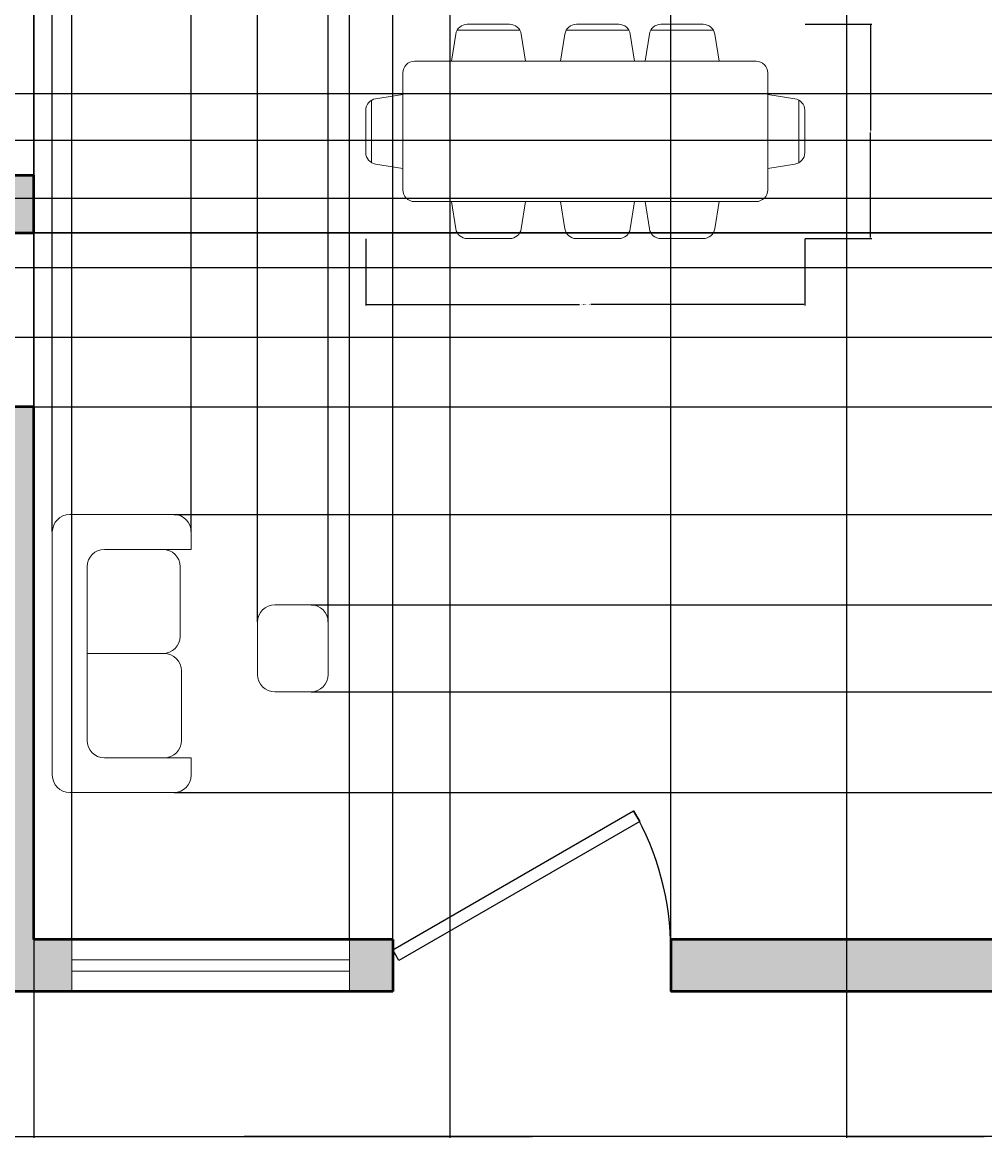
# Model space of a CAD drawing. Units: inches. Extents: x 3439 to 3988, y 1915 to 2284.
# Tile 4 of 7: x 3656 to 3822, y 1915 to 2108. Entities that reach past the tile are written whole.
import ezdxf

# ---------------------------------------------------------------- set-up
doc = ezdxf.new("R2010")
doc.units = ezdxf.units.IN
for name, color, linetype, lineweight in [('A-ANNO-DIMS', 2, 'Continuous', 18), ('A-DOOR', 3, 'Continuous', 25), ('A-FURN', 9, 'Continuous', 18), ('A-GLAZ', 4, 'Continuous', 18), ('A-WALL', 7, 'Continuous', 50)]:
    doc.layers.add(name, color=color, linetype=linetype, lineweight=lineweight)
doc.layers.add('A-WALL-PATT', color=18, linetype='Continuous', lineweight=13, true_color=0x000000)
doc.styles.get("Standard").update_dxf_attribs({"font": 'arial.ttf'})
doc.dimstyles.get("Standard").update_dxf_attribs({"dimtxt": 0.18, "dimasz": 0.18, "dimexe": 0.18, "dimexo": 0.0625, "dimgap": 0.09, "dimtad": 0, "dimtih": 1, "dimtoh": 1, "dimdec": 4, "dimzin": 0, "dimdsep": 46, "dimtxsty": 'Standard', "dimcen": 0.09, "dimadec": 0, "dimazin": 0, "dimtfac": 1, "dimtdec": 4, "dimtofl": 0, "dimtmove": 0, "dimatfit": 3, "dimfxl": 1, "dimtolj": 1, "dimtzin": 0, "dimarcsym": 0})

# ---------------------------------------------------------------- blocks, each defined once
blk = doc.blocks.new('*U4')
for p, q in [((0, 0), (0, -6)), ((40, 0), (40, -6))]:
    blk.add_line(p, q)
blk.add_lwpolyline([(0, 0), (34.64, 20), (35.52, 18.48), (0.87, -1.52)], close=True)
blk.add_arc((0, 0), 40, 0, 30)
blk = doc.blocks.new('*U5')
for p, q in [((0, 0), (0, 6)), ((40, 0), (40, 6))]:
    blk.add_line(p, q)
blk.add_lwpolyline([(0, 0), (34.64, -20), (35.52, -18.48), (0.87, 1.52)], close=True)
blk.add_arc((0, 0), 40, 330, 0)
blk = doc.blocks.new('Dining Set - 36 x 72 in.')
for p, q in [((-22.03, 26), (-5.97, 26)), ((-19.43, 27.5), (-8.57, 27.5)), ((5.97, 26), (22.03, 26)), ((8.57, 27.5), (19.43, 27.5)), ((27.65, 26), (43.71, 26)), ((30.25, 27.5), (41.11, 27.5)), ((-22.4, 24.96), (-23.48, 18)), ((-4.52, 18), (-5.6, 24.96)), ((5.6, 24.96), (4.52, 18)), ((23.48, 18), (22.4, 24.96)), ((27.29, 24.96), (26.2, 18)), ((45.17, 18), (44.08, 24.96)), ((3.02, 18), (-33, 18)), ((3.02, 18), (24.7, 18)), ((23.48, 18), (4.52, 18)), ((24.7, 18), (46.38, 18)), ((45.17, 18), (26.2, 18)), ((54.68, 18), (46.38, 18)), ((-36, 15), (-36, -15)), ((57.68, -15), (57.68, 15)), ((-42.96, 8.4), (-36, 9.48)), ((64.64, 8.4), (57.68, 9.48)), ((-44, 8.03), (-44, -8.03)), ((65.68, 8.03), (65.68, -8.03)), ((-45.5, 5.43), (-45.5, -5.43)), ((67.18, 5.43), (67.18, -5.43)), ((-36, -9.48), (-42.96, -8.4)), ((57.68, -9.48), (64.64, -8.4)), ((-33, -18), (3.02, -18)), ((-22.4, -24.96), (-23.48, -18)), ((-4.52, -18), (-5.6, -24.96)), ((3.02, -18), (24.7, -18)), ((4.52, -18), (23.48, -18)), ((5.6, -24.96), (4.52, -18)), ((23.48, -18), (22.4, -24.96)), ((24.7, -18), (46.38, -18)), ((27.29, -24.96), (26.2, -18)), ((26.2, -18), (45.17, -18)), ((45.17, -18), (44.08, -24.96)), ((46.38, -18), (54.68, -18)), ((-22.03, -26), (-5.97, -26)), ((-19.43, -27.5), (-8.57, -27.5)), ((5.97, -26), (22.03, -26)), ((8.57, -27.5), (19.43, -27.5)), ((27.65, -26), (43.71, -26)), ((30.25, -27.5), (41.11, -27.5))]:
    blk.add_line(p, q)
for centre, start, end in [((-19.43, 24.5), 90, 171.1198), ((-8.57, 24.5), 8.881, 90), ((8.57, 24.5), 90, 171.1198), ((19.43, 24.5), 8.881, 90), ((30.25, 24.5), 90, 171.1198), ((41.11, 24.5), 8.881, 90), ((-33, 15), 90, 180), ((54.68, 15), 0, 90), ((-42.5, 5.43), 98.8806, 180), ((64.18, 5.43), 0, 81.1194), ((-42.5, -5.43), 180, 261.1194), ((64.18, -5.43), 278.8806, 0), ((-33, -15), 180, 270), ((54.68, -15), 270, 0), ((-19.43, -24.5), 188.8802, 270), ((-8.57, -24.5), 270, 351.1191), ((8.57, -24.5), 188.8802, 270), ((19.43, -24.5), 270, 351.1191), ((30.25, -24.5), 188.8802, 270), ((41.11, -24.5), 270, 351.1191)]:
    blk.add_arc(centre, 3, start, end)
blk = doc.blocks.new('WINDOW-GLASS-48IN')
for p, q in [((0, 2), (48, 2)), ((0, 0), (48, 0))]:
    blk.add_line(p, q)
blk = doc.blocks.new('*D41')
at = {"layer": 'A-ANNO-DIMS', "color": 0, "lineweight": -2, "transparency": 16777216}
for p, q in [((3714.9, 2070.32), (3714.9, 2058.83)), ((3790.73, 2070.32), (3790.73, 2058.83)), ((3715.08, 2059.01), (3751.84, 2059.01)), ((3790.55, 2059.01), (3753.78, 2059.01))]:
    blk.add_line(p, q, dxfattribs=at)
at = {"layer": 'A-ANNO-DIMS', "color": 0, "transparency": 16777216}
for points in [[(3715.08, 2059.04), (3715.08, 2058.98), (3714.9, 2059.01)], [(3790.55, 2059.04), (3790.55, 2058.98), (3790.73, 2059.01)]]:
    blk.add_solid(points, dxfattribs=at)
at = {"layer": 'Defpoints', "color": 0, "transparency": 16777216}
for p in [(3714.9, 2070.38), (3790.73, 2070.38), (3790.73, 2059.01)]:
    blk.add_point(p, dxfattribs=at)
at = {"layer": 'A-ANNO-DIMS', "color": 0, "transparency": 16777216, "insert": (3752.81, 2059.01), "char_height": 0.18, "attachment_point": 5}
blk.add_mtext('\\A1;DINING SET 76', dxfattribs=at)
blk = doc.blocks.new('*D42')
at = {"layer": 'A-ANNO-DIMS', "color": 0, "lineweight": -2, "transparency": 16777216}
for p, q in [((3790.79, 2107.39), (3802.28, 2107.39)), ((3802.1, 2107.21), (3802.1, 2089.07)), ((3802.1, 2070.56), (3802.1, 2088.7)), ((3790.79, 2070.38), (3802.28, 2070.38))]:
    blk.add_line(p, q, dxfattribs=at)
at = {"layer": 'A-ANNO-DIMS', "color": 0, "transparency": 16777216}
for points in [[(3802.07, 2107.21), (3802.13, 2107.21), (3802.1, 2107.39)], [(3802.07, 2070.56), (3802.13, 2070.56), (3802.1, 2070.38)]]:
    blk.add_solid(points, dxfattribs=at)
at = {"layer": 'Defpoints', "color": 0, "transparency": 16777216}
for p in [(3790.73, 2107.39), (3802.1, 2107.39), (3790.73, 2070.38)]:
    blk.add_point(p, dxfattribs=at)
at = {"layer": 'A-ANNO-DIMS', "color": 0, "transparency": 16777216, "insert": (3802.1, 2088.89), "char_height": 0.18, "attachment_point": 5}
blk.add_mtext('\\A1;37', dxfattribs=at)
blk = doc.blocks.new('*D45')
at = {"layer": 'A-ANNO-DIMS', "color": 0, "lineweight": -2, "transparency": 16777216}
for p, q in [((3464.58, 1940.3), (3464.58, 1915.13)), ((3962.58, 1940.3), (3962.58, 1915.13)), ((3464.76, 1915.31), (3713.29, 1915.31)), ((3962.4, 1915.31), (3713.87, 1915.31))]:
    blk.add_line(p, q, dxfattribs=at)
at = {"layer": 'A-ANNO-DIMS', "color": 0, "transparency": 16777216}
for points in [[(3464.76, 1915.34), (3464.76, 1915.28), (3464.58, 1915.31)], [(3962.4, 1915.34), (3962.4, 1915.28), (3962.58, 1915.31)]]:
    blk.add_solid(points, dxfattribs=at)
at = {"layer": 'Defpoints', "color": 0, "transparency": 16777216}
for p in [(3464.58, 1940.36), (3962.58, 1940.36), (3962.58, 1915.31)]:
    blk.add_point(p, dxfattribs=at)
at = {"layer": 'A-ANNO-DIMS', "color": 0, "transparency": 16777216, "insert": (3713.58, 1915.31), "char_height": 0.18, "attachment_point": 5}
blk.add_mtext('\\A1;498', dxfattribs=at)
blk = doc.blocks.new('*D50')
at = {"layer": 'A-ANNO-DIMS', "color": 0, "lineweight": -2, "transparency": 16777216}
for p, q in [((3797.93, 2249.3), (3797.93, 1915.13)), ((3845.93, 2249.3), (3845.93, 1915.13)), ((3798.11, 1915.31), (3821.71, 1915.31)), ((3845.75, 1915.31), (3822.15, 1915.31))]:
    blk.add_line(p, q, dxfattribs=at)
at = {"layer": 'A-ANNO-DIMS', "color": 0, "transparency": 16777216}
for points in [[(3798.11, 1915.34), (3798.11, 1915.28), (3797.93, 1915.31)], [(3845.75, 1915.34), (3845.75, 1915.28), (3845.93, 1915.31)]]:
    blk.add_solid(points, dxfattribs=at)
at = {"layer": 'Defpoints', "color": 0, "transparency": 16777216}
for p in [(3797.93, 2249.36), (3845.93, 2249.36), (3845.93, 1915.31)]:
    blk.add_point(p, dxfattribs=at)
at = {"layer": 'A-ANNO-DIMS', "color": 0, "transparency": 16777216, "insert": (3821.93, 1915.31), "char_height": 0.18, "attachment_point": 5}
blk.add_mtext('\\A1;48', dxfattribs=at)
blk = doc.blocks.new('*D53')
at = {"layer": 'A-ANNO-DIMS', "color": 0, "lineweight": -2, "transparency": 16777216}
for p, q in [((3829.58, 2065.3), (3829.58, 1915.13)), ((3657.58, 2041.3), (3657.58, 1915.13)), ((3657.76, 1915.31), (3743.3, 1915.31)), ((3829.4, 1915.31), (3743.86, 1915.31))]:
    blk.add_line(p, q, dxfattribs=at)
at = {"layer": 'A-ANNO-DIMS', "color": 0, "transparency": 16777216}
for points in [[(3657.76, 1915.34), (3657.76, 1915.28), (3657.58, 1915.31)], [(3829.4, 1915.34), (3829.4, 1915.28), (3829.58, 1915.31)]]:
    blk.add_solid(points, dxfattribs=at)
at = {"layer": 'Defpoints', "color": 0, "transparency": 16777216}
for p in [(3829.58, 2065.36), (3657.58, 2041.36), (3829.58, 1915.31)]:
    blk.add_point(p, dxfattribs=at)
at = {"layer": 'A-ANNO-DIMS', "color": 0, "transparency": 16777216, "insert": (3743.58, 1915.31), "char_height": 0.18, "attachment_point": 5}
blk.add_mtext('\\A1;172', dxfattribs=at)
blk = doc.blocks.new('*D62')
at = {"layer": 'A-ANNO-DIMS', "color": 0, "lineweight": -2, "transparency": 16777216}
for p, q in [((3537.64, 2077.36), (3987.81, 2077.36)), ((3987.63, 2077.18), (3987.63, 2065.54)), ((3987.63, 2053.54), (3987.63, 2065.18)), ((3537.64, 2053.36), (3987.81, 2053.36))]:
    blk.add_line(p, q, dxfattribs=at)
at = {"layer": 'A-ANNO-DIMS', "color": 0, "transparency": 16777216}
for points in [[(3987.6, 2077.18), (3987.66, 2077.18), (3987.63, 2077.36)], [(3987.6, 2053.54), (3987.66, 2053.54), (3987.63, 2053.36)]]:
    blk.add_solid(points, dxfattribs=at)
at = {"layer": 'Defpoints', "color": 0, "transparency": 16777216}
for p in [(3537.58, 2077.36), (3987.63, 2077.36), (3537.58, 2053.36)]:
    blk.add_point(p, dxfattribs=at)
at = {"layer": 'A-ANNO-DIMS', "color": 0, "transparency": 16777216, "insert": (3987.63, 2065.36), "char_height": 0.18, "attachment_point": 5}
blk.add_mtext('\\A1;24', dxfattribs=at)
blk = doc.blocks.new('*D73')
at = {"layer": 'A-ANNO-DIMS', "color": 0, "lineweight": -2, "transparency": 16777216}
for p, q in [((3657.58, 1949.42), (3657.58, 2284)), ((3657.76, 2283.82), (3660.52, 2283.82)), ((3663.93, 2283.82), (3661.17, 2283.82)), ((3664.11, 1949.42), (3664.11, 2284))]:
    blk.add_line(p, q, dxfattribs=at)
at = {"layer": 'A-ANNO-DIMS', "color": 0, "transparency": 16777216}
for points in [[(3657.76, 2283.85), (3657.76, 2283.79), (3657.58, 2283.82)], [(3663.93, 2283.85), (3663.93, 2283.79), (3664.11, 2283.82)]]:
    blk.add_solid(points, dxfattribs=at)
at = {"layer": 'Defpoints', "color": 0, "transparency": 16777216}
for p in [(3664.11, 2283.82), (3657.58, 1949.36), (3664.11, 1949.36)]:
    blk.add_point(p, dxfattribs=at)
at = {"layer": 'A-ANNO-DIMS', "color": 0, "transparency": 16777216, "insert": (3660.85, 2283.82), "char_height": 0.18, "attachment_point": 5}
blk.add_mtext('\\A1;6.53', dxfattribs=at)
blk = doc.blocks.new('*D74')
at = {"layer": 'A-ANNO-DIMS', "color": 0, "lineweight": -2, "transparency": 16777216}
for p, q in [((3712.11, 1949.42), (3712.11, 2284)), ((3712.29, 2283.82), (3715.52, 2283.82)), ((3719.4, 2283.82), (3716.17, 2283.82)), ((3719.58, 1949.42), (3719.58, 2284))]:
    blk.add_line(p, q, dxfattribs=at)
at = {"layer": 'A-ANNO-DIMS', "color": 0, "transparency": 16777216}
for points in [[(3712.29, 2283.85), (3712.29, 2283.79), (3712.11, 2283.82)], [(3719.4, 2283.85), (3719.4, 2283.79), (3719.58, 2283.82)]]:
    blk.add_solid(points, dxfattribs=at)
at = {"layer": 'Defpoints', "color": 0, "transparency": 16777216}
for p in [(3719.58, 2283.82), (3712.11, 1949.36), (3719.58, 1949.36)]:
    blk.add_point(p, dxfattribs=at)
at = {"layer": 'A-ANNO-DIMS', "color": 0, "transparency": 16777216, "insert": (3715.85, 2283.82), "char_height": 0.18, "attachment_point": 5}
blk.add_mtext('\\A1;7.47', dxfattribs=at)
blk = doc.blocks.new('*D75')
at = {"layer": 'A-ANNO-DIMS', "color": 0, "lineweight": -2, "transparency": 16777216}
for p, q in [((3719.58, 1949.42), (3719.58, 2284)), ((3719.76, 2283.82), (3743.36, 2283.82)), ((3767.4, 2283.82), (3743.8, 2283.82)), ((3767.58, 1949.42), (3767.58, 2284))]:
    blk.add_line(p, q, dxfattribs=at)
at = {"layer": 'A-ANNO-DIMS', "color": 0, "transparency": 16777216}
for points in [[(3719.76, 2283.85), (3719.76, 2283.79), (3719.58, 2283.82)], [(3767.4, 2283.85), (3767.4, 2283.79), (3767.58, 2283.82)]]:
    blk.add_solid(points, dxfattribs=at)
at = {"layer": 'Defpoints', "color": 0, "transparency": 16777216}
for p in [(3767.58, 2283.82), (3719.58, 1949.36), (3767.58, 1949.36)]:
    blk.add_point(p, dxfattribs=at)
at = {"layer": 'A-ANNO-DIMS', "color": 0, "transparency": 16777216, "insert": (3743.58, 2283.82), "char_height": 0.18, "attachment_point": 5}
blk.add_mtext('\\A1;48', dxfattribs=at)
blk = doc.blocks.new('*D83')
at = {"layer": 'A-ANNO-DIMS', "color": 0, "lineweight": -2, "transparency": 16777216}
for p, q in [((3537.64, 2111.36), (3987.81, 2111.36)), ((3987.63, 2111.18), (3987.63, 2099.54)), ((3987.63, 2087.54), (3987.63, 2099.18)), ((3537.64, 2087.36), (3987.81, 2087.36))]:
    blk.add_line(p, q, dxfattribs=at)
at = {"layer": 'A-ANNO-DIMS', "color": 0, "transparency": 16777216}
for points in [[(3987.6, 2111.18), (3987.66, 2111.18), (3987.63, 2111.36)], [(3987.6, 2087.54), (3987.66, 2087.54), (3987.63, 2087.36)]]:
    blk.add_solid(points, dxfattribs=at)
at = {"layer": 'Defpoints', "color": 0, "transparency": 16777216}
for p in [(3537.58, 2111.36), (3987.63, 2111.36), (3537.58, 2087.36)]:
    blk.add_point(p, dxfattribs=at)
at = {"layer": 'A-ANNO-DIMS', "color": 0, "transparency": 16777216, "insert": (3987.63, 2099.36), "char_height": 0.18, "attachment_point": 5}
blk.add_mtext('\\A1;24', dxfattribs=at)
blk = doc.blocks.new('*D88')
at = {"layer": 'A-ANNO-DIMS', "color": 0, "lineweight": -2, "transparency": 16777216}
for p, q in [((3653.64, 2077.36), (3987.81, 2077.36)), ((3987.63, 2077.18), (3987.63, 2074.54)), ((3987.63, 2071.54), (3987.63, 2074.18)), ((3653.64, 2071.36), (3987.81, 2071.36))]:
    blk.add_line(p, q, dxfattribs=at)
at = {"layer": 'A-ANNO-DIMS', "color": 0, "transparency": 16777216}
for points in [[(3987.6, 2077.18), (3987.66, 2077.18), (3987.63, 2077.36)], [(3987.6, 2071.54), (3987.66, 2071.54), (3987.63, 2071.36)]]:
    blk.add_solid(points, dxfattribs=at)
at = {"layer": 'Defpoints', "color": 0, "transparency": 16777216}
for p in [(3653.58, 2077.36), (3987.63, 2077.36), (3653.58, 2071.36)]:
    blk.add_point(p, dxfattribs=at)
at = {"layer": 'A-ANNO-DIMS', "color": 0, "transparency": 16777216, "insert": (3987.63, 2074.36), "char_height": 0.18, "attachment_point": 5}
blk.add_mtext('\\A1;6', dxfattribs=at)
blk = doc.blocks.new('*D89')
at = {"layer": 'A-ANNO-DIMS', "color": 0, "lineweight": -2, "transparency": 16777216}
for p, q in [((3657.64, 2071.36), (3987.81, 2071.36)), ((3987.63, 2071.18), (3987.63, 2056.54)), ((3987.63, 2041.54), (3987.63, 2056.18)), ((3657.64, 2041.36), (3987.81, 2041.36))]:
    blk.add_line(p, q, dxfattribs=at)
at = {"layer": 'A-ANNO-DIMS', "color": 0, "transparency": 16777216}
for points in [[(3987.6, 2071.18), (3987.66, 2071.18), (3987.63, 2071.36)], [(3987.6, 2041.54), (3987.66, 2041.54), (3987.63, 2041.36)]]:
    blk.add_solid(points, dxfattribs=at)
at = {"layer": 'Defpoints', "color": 0, "transparency": 16777216}
for p in [(3657.58, 2071.36), (3987.63, 2071.36), (3657.58, 2041.36)]:
    blk.add_point(p, dxfattribs=at)
at = {"layer": 'A-ANNO-DIMS', "color": 0, "transparency": 16777216, "insert": (3987.63, 2056.36), "char_height": 0.18, "attachment_point": 5}
blk.add_mtext('\\A1;30', dxfattribs=at)
blk = doc.blocks.new('*D90')
at = {"layer": 'A-ANNO-DIMS', "color": 0, "lineweight": -2, "transparency": 16777216}
for p, q in [((3889.52, 2071.36), (3439.35, 2071.36)), ((3439.53, 2071.18), (3439.53, 2068.54)), ((3439.53, 2065.54), (3439.53, 2068.18)), ((3889.52, 2065.36), (3439.35, 2065.36))]:
    blk.add_line(p, q, dxfattribs=at)
at = {"layer": 'A-ANNO-DIMS', "color": 0, "transparency": 16777216}
for points in [[(3439.5, 2071.18), (3439.56, 2071.18), (3439.53, 2071.36)], [(3439.5, 2065.54), (3439.56, 2065.54), (3439.53, 2065.36)]]:
    blk.add_solid(points, dxfattribs=at)
at = {"layer": 'Defpoints', "color": 0, "transparency": 16777216}
for p in [(3439.53, 2071.36), (3889.58, 2071.36), (3889.58, 2065.36)]:
    blk.add_point(p, dxfattribs=at)
at = {"layer": 'A-ANNO-DIMS', "color": 0, "transparency": 16777216, "insert": (3439.53, 2068.36), "char_height": 0.18, "attachment_point": 5}
blk.add_mtext('\\A1;6', dxfattribs=at)
blk = doc.blocks.new('*D91')
at = {"layer": 'A-ANNO-DIMS', "color": 0, "lineweight": -2, "transparency": 16777216}
for p, q in [((3889.52, 2095.36), (3439.35, 2095.36)), ((3439.53, 2095.18), (3439.53, 2083.54)), ((3439.53, 2071.54), (3439.53, 2083.18)), ((3889.52, 2071.36), (3439.35, 2071.36))]:
    blk.add_line(p, q, dxfattribs=at)
at = {"layer": 'A-ANNO-DIMS', "color": 0, "transparency": 16777216}
for points in [[(3439.5, 2095.18), (3439.56, 2095.18), (3439.53, 2095.36)], [(3439.5, 2071.54), (3439.56, 2071.54), (3439.53, 2071.36)]]:
    blk.add_solid(points, dxfattribs=at)
at = {"layer": 'Defpoints', "color": 0, "transparency": 16777216}
for p in [(3439.53, 2095.36), (3889.58, 2095.36), (3889.58, 2071.36)]:
    blk.add_point(p, dxfattribs=at)
at = {"layer": 'A-ANNO-DIMS', "color": 0, "transparency": 16777216, "insert": (3439.53, 2083.36), "char_height": 0.18, "attachment_point": 5}
blk.add_mtext('\\A1;24', dxfattribs=at)
blk = doc.blocks.new('*D92')
at = {"layer": 'A-ANNO-DIMS', "color": 0, "lineweight": -2, "transparency": 16777216}
for p, q in [((3767.64, 1949.36), (3987.81, 1949.36)), ((3987.63, 1949.18), (3987.63, 1945.04)), ((3987.63, 1940.54), (3987.63, 1944.68)), ((3767.64, 1940.36), (3987.81, 1940.36))]:
    blk.add_line(p, q, dxfattribs=at)
at = {"layer": 'A-ANNO-DIMS', "color": 0, "transparency": 16777216}
for points in [[(3987.6, 1949.18), (3987.66, 1949.18), (3987.63, 1949.36)], [(3987.6, 1940.54), (3987.66, 1940.54), (3987.63, 1940.36)]]:
    blk.add_solid(points, dxfattribs=at)
at = {"layer": 'Defpoints', "color": 0, "transparency": 16777216}
for p in [(3767.58, 1949.36), (3987.63, 1949.36), (3767.58, 1940.36)]:
    blk.add_point(p, dxfattribs=at)
at = {"layer": 'A-ANNO-DIMS', "color": 0, "transparency": 16777216, "insert": (3987.63, 1944.86), "char_height": 0.18, "attachment_point": 5}
blk.add_mtext('\\A1;9', dxfattribs=at)
blk = doc.blocks.new('*D94')
at = {"layer": 'A-ANNO-DIMS', "color": 0, "lineweight": -2, "transparency": 16777216}
for p, q in [((3657.58, 2141.3), (3657.58, 1915.13)), ((3729.41, 2141.3), (3729.41, 1915.13)), ((3657.76, 1915.31), (3693.1, 1915.31)), ((3729.23, 1915.31), (3693.89, 1915.31))]:
    blk.add_line(p, q, dxfattribs=at)
at = {"layer": 'A-ANNO-DIMS', "color": 0, "transparency": 16777216}
for points in [[(3657.76, 1915.34), (3657.76, 1915.28), (3657.58, 1915.31)], [(3729.23, 1915.34), (3729.23, 1915.28), (3729.41, 1915.31)]]:
    blk.add_solid(points, dxfattribs=at)
at = {"layer": 'Defpoints', "color": 0, "transparency": 16777216}
for p in [(3657.58, 2141.36), (3729.41, 2141.36), (3729.41, 1915.31)]:
    blk.add_point(p, dxfattribs=at)
at = {"layer": 'A-ANNO-DIMS', "color": 0, "transparency": 16777216, "insert": (3693.49, 1915.31), "char_height": 0.18, "attachment_point": 5}
blk.add_mtext('\\A1;71.83', dxfattribs=at)
blk = doc.blocks.new('*D99')
at = {"layer": 'A-ANNO-DIMS', "color": 0, "lineweight": -2, "transparency": 16777216}
for p, q in [((3660.76, 2019.79), (3660.76, 2284)), ((3660.94, 2283.82), (3672.54, 2283.82)), ((3684.58, 2283.82), (3672.98, 2283.82)), ((3684.76, 2019.79), (3684.76, 2284))]:
    blk.add_line(p, q, dxfattribs=at)
at = {"layer": 'A-ANNO-DIMS', "color": 0, "transparency": 16777216}
for points in [[(3660.94, 2283.85), (3660.94, 2283.79), (3660.76, 2283.82)], [(3684.58, 2283.85), (3684.58, 2283.79), (3684.76, 2283.82)]]:
    blk.add_solid(points, dxfattribs=at)
at = {"layer": 'Defpoints', "color": 0, "transparency": 16777216}
for p in [(3684.76, 2283.82), (3660.76, 2019.72), (3684.76, 2019.72)]:
    blk.add_point(p, dxfattribs=at)
at = {"layer": 'A-ANNO-DIMS', "color": 0, "transparency": 16777216, "insert": (3672.76, 2283.82), "char_height": 0.18, "attachment_point": 5}
blk.add_mtext('\\A1;24', dxfattribs=at)
blk = doc.blocks.new('*D100')
at = {"layer": 'A-ANNO-DIMS', "color": 0, "lineweight": -2, "transparency": 16777216}
for p, q in [((3681.83, 2022.72), (3987.81, 2022.72)), ((3987.63, 2022.54), (3987.63, 1998.91)), ((3987.63, 1974.9), (3987.63, 1998.54)), ((3681.83, 1974.72), (3987.81, 1974.72))]:
    blk.add_line(p, q, dxfattribs=at)
at = {"layer": 'A-ANNO-DIMS', "color": 0, "transparency": 16777216}
for points in [[(3987.6, 2022.54), (3987.66, 2022.54), (3987.63, 2022.72)], [(3987.6, 1974.9), (3987.66, 1974.9), (3987.63, 1974.72)]]:
    blk.add_solid(points, dxfattribs=at)
at = {"layer": 'Defpoints', "color": 0, "transparency": 16777216}
for p in [(3681.76, 2022.72), (3987.63, 2022.72), (3681.76, 1974.72)]:
    blk.add_point(p, dxfattribs=at)
at = {"layer": 'A-ANNO-DIMS', "color": 0, "transparency": 16777216, "insert": (3987.63, 1998.72), "char_height": 0.18, "attachment_point": 5}
blk.add_mtext('\\A1;48', dxfattribs=at)
blk = doc.blocks.new('*D101')
at = {"layer": 'A-ANNO-DIMS', "color": 0, "lineweight": -2, "transparency": 16777216}
for p, q in [((3696.21, 2004.22), (3696.21, 2284)), ((3696.39, 2283.82), (3701.86, 2283.82)), ((3708.24, 2283.82), (3702.77, 2283.82)), ((3708.42, 2004.22), (3708.42, 2284))]:
    blk.add_line(p, q, dxfattribs=at)
at = {"layer": 'A-ANNO-DIMS', "color": 0, "transparency": 16777216}
for points in [[(3696.39, 2283.85), (3696.39, 2283.79), (3696.21, 2283.82)], [(3708.24, 2283.85), (3708.24, 2283.79), (3708.42, 2283.82)]]:
    blk.add_solid(points, dxfattribs=at)
at = {"layer": 'Defpoints', "color": 0, "transparency": 16777216}
for p in [(3708.42, 2283.82), (3696.21, 2004.16), (3708.42, 2004.16)]:
    blk.add_point(p, dxfattribs=at)
at = {"layer": 'A-ANNO-DIMS', "color": 0, "transparency": 16777216, "insert": (3702.31, 2283.82), "char_height": 0.18, "attachment_point": 5}
blk.add_mtext('\\A1;12.214', dxfattribs=at)
blk = doc.blocks.new('*D102')
at = {"layer": 'A-ANNO-DIMS', "color": 0, "lineweight": -2, "transparency": 16777216}
for p, q in [((3705.48, 2007.16), (3987.81, 2007.16)), ((3987.63, 2006.98), (3987.63, 1999.83)), ((3987.63, 1992.31), (3987.63, 1999.46)), ((3705.48, 1992.13), (3987.81, 1992.13))]:
    blk.add_line(p, q, dxfattribs=at)
at = {"layer": 'A-ANNO-DIMS', "color": 0, "transparency": 16777216}
for points in [[(3987.6, 2006.98), (3987.66, 2006.98), (3987.63, 2007.16)], [(3987.6, 1992.31), (3987.66, 1992.31), (3987.63, 1992.13)]]:
    blk.add_solid(points, dxfattribs=at)
at = {"layer": 'Defpoints', "color": 0, "transparency": 16777216}
for p in [(3705.42, 2007.16), (3987.63, 2007.16), (3705.42, 1992.13)]:
    blk.add_point(p, dxfattribs=at)
at = {"layer": 'A-ANNO-DIMS', "color": 0, "transparency": 16777216, "insert": (3987.63, 1999.64), "char_height": 0.18, "attachment_point": 5}
blk.add_mtext('\\A1;15.025', dxfattribs=at)

msp = doc.modelspace()

# ---------------------------------------------------------------- hatches: boundary and pattern name
at = {"layer": 'A-WALL-PATT'}
h = msp.add_hatch(color=256, dxfattribs=at)
h.dxf.hatch_style = 1
h.paths.add_polyline_path([(3551.6168, 1949.3617), (3473.5815, 1949.3617), (3473.5815, 2053.3617), (3537.5815, 2053.3617), (3537.5815, 2077.3617), (3653.5815, 2077.3617), (3653.5815, 2071.3617), (3657.5815, 2071.3617), (3657.5815, 2081.3617), (3537.5815, 2081.3617), (3537.5815, 2087.3617), (3533.5815, 2087.3617), (3533.5815, 2057.3617), (3473.5815, 2057.3617), (3473.5815, 2084.0664), (3464.5815, 2084.0664), (3464.5815, 1940.3617), (3551.6168, 1940.3617)])
h = msp.add_hatch(color=256, dxfattribs=at)
h.dxf.hatch_style = 1
h.paths.add_polyline_path([(3865.0815, 1949.3617), (3833.5815, 1949.3617), (3833.5815, 2061.3617), (3839.5815, 2061.3617), (3839.5815, 2065.3617), (3829.5815, 2065.3617), (3829.5815, 1949.3617), (3767.5815, 1949.3617), (3767.5815, 1940.3617), (3865.0815, 1940.3617)])
h = msp.add_hatch(color=256, dxfattribs=at)
h.dxf.hatch_style = 1
h.paths.add_polyline_path([(3664.1118, 1949.3617), (3657.5815, 1949.3617), (3657.5815, 2041.3617), (3653.5815, 2041.3617), (3653.5815, 1949.3617), (3599.6168, 1949.3617), (3599.6168, 1940.3617), (3664.1118, 1940.3617)])
h = msp.add_hatch(color=256, dxfattribs=at)
h.dxf.hatch_style = 1
h.paths.add_polyline_path([(3719.5815, 1947.5617), (3719.5815, 1949.3617), (3712.1118, 1949.3617), (3712.1118, 1940.3617), (3719.5815, 1940.3617)])

# ---------------------------------------------------------------- linework, layer by layer
at = {"layer": 'A-FURN'}
for p, q in [((3663.7646, 2022.7238), (3681.7646, 2022.7238)), ((3660.7646, 2019.7238), (3660.7646, 1977.7238)), ((3684.7646, 2019.7238), (3684.7646, 2016.7238)), ((3669.7646, 2016.7238), (3684.7646, 2016.7238)), ((3666.7646, 2013.7238), (3666.7646, 1983.7238)), ((3669.7646, 1980.7238), (3684.7646, 1980.7238)), ((3684.7646, 1980.7238), (3684.7646, 1977.7238)), ((3663.7646, 1974.7238), (3681.7646, 1974.7238))]:
    msp.add_line(p, q, dxfattribs=at)
for points in [[(3669.7646, 2016.7238), (3679.8502, 2016.7238, -0.41421356), (3682.8502, 2013.7238), (3682.8502, 2001.7238, -0.41421356), (3679.8502, 1998.7238), (3666.7646, 1998.7238), (3666.7646, 2013.7238, -0.41421356)], [(3699.2076, 2007.1572), (3705.4216, 2007.1572, -0.41421356), (3708.4216, 2004.1572), (3708.4216, 1995.1326, -0.41421356), (3705.4216, 1992.1326), (3699.2076, 1992.1326, -0.41421356), (3696.2076, 1995.1326), (3696.2076, 2004.1572, -0.41421356)], [(3666.7646, 1998.7238), (3680.0639, 1998.7238, -0.41421356), (3683.0639, 1995.7238), (3683.0639, 1983.7238, -0.41421356), (3680.0639, 1980.7238), (3669.7646, 1980.7238, -0.41421356), (3666.7646, 1983.7238)]]:
    msp.add_lwpolyline(points, format="xyb", close=True, dxfattribs=at)
for centre, start, end in [((3663.7646, 2019.7238), 90, 180), ((3681.7646, 2019.7238), 0, 90), ((3669.7646, 2013.7238), 90, 180), ((3669.7646, 1983.7238), 180, 270), ((3663.7646, 1977.7238), 180, 270), ((3681.7646, 1977.7238), 270, 0)]:
    msp.add_arc(centre, 3, start, end, dxfattribs=at)
at = {"layer": 'A-GLAZ'}
for points in [[(3664.1118, 1940.3617), (3664.1118, 1949.3617)], [(3712.1118, 1949.3617), (3712.1118, 1940.3617)]]:
    msp.add_lwpolyline(points, dxfattribs=at)
at = {"layer": 'A-WALL'}
for p, q in [((3537.5815, 2081.3617), (3657.5815, 2081.3617)), ((3657.5815, 2071.3617), (3657.5815, 2081.3617)), ((3653.5815, 2071.3617), (3657.5815, 2071.3617)), ((3653.5815, 2041.3617), (3657.5815, 2041.3617)), ((3657.5815, 1949.3617), (3657.5815, 2041.3617)), ((3719.5815, 1949.3617), (3657.5815, 1949.3617)), ((3719.5815, 1949.3617), (3719.5815, 1940.3617)), ((3829.5815, 1949.3617), (3767.5815, 1949.3617)), ((3767.5815, 1949.3617), (3767.5815, 1940.3617))]:
    msp.add_line(p, q, dxfattribs=at)
for points in [[(3719.5815, 1940.3617), (3464.5815, 1940.3617), (3464.5815, 2258.3617), (3803.9319, 2258.3617)], [(3827.9319, 2258.3617), (3962.5815, 2258.3617), (3962.5815, 1940.3617), (3767.5815, 1940.3617)]]:
    msp.add_lwpolyline(points, dxfattribs=at)

# ---------------------------------------------------------------- block references
at = {"layer": 'A-DOOR', "xscale": 0.75, "yscale": 0.75, "zscale": 0.75, "rotation": 270}
msp.add_blockref('*U5', (3653.0815, 2071.3617), dxfattribs=at)
at = {"layer": 'A-DOOR', "xscale": 1.199999999999999, "yscale": 1.199999999999999, "zscale": 1.199999999999999}
msp.add_blockref('*U4', (3719.5815, 1947.5617), dxfattribs=at)
at = {"layer": 'A-FURN', "xscale": 0.672937641053352, "yscale": 0.672937641053352, "zscale": 0.672937641053352}
msp.add_blockref('Dining Set - 36 x 72 in.', (3745.5162, 2088.8854), dxfattribs=at)
at = {"layer": 'A-GLAZ'}
msp.add_blockref('WINDOW-GLASS-48IN', (3664.1118, 1943.8617), dxfattribs=at)

# ---------------------------------------------------------------- dimensions: what is measured, and where the dimension line sits
at = {"layer": 'A-ANNO-DIMS'}
for base, p1, p2, override, picture, middle in [((3664.1118, 2283.8228), (3657.5815, 1949.3617), (3664.1118, 1949.3617), {"dimdec": 2, "dimlfac": 1, "dimrnd": 0, "dimzin": 0, "dimdsep": 46, "dimlunit": 2}, '*D73', (3660.8466, 2283.8228)), ((3684.7646, 2283.8228), (3660.7646, 2019.7238), (3684.7646, 2019.7238), {"dimdec": 0, "dimlfac": 1, "dimrnd": 0, "dimzin": 0, "dimdsep": 46, "dimlunit": 2}, '*D99', (3672.7646, 2283.8228)), ((3708.4216, 2283.8228), (3696.2076, 2004.1572), (3708.4216, 2004.1572), {"dimdec": 3, "dimlfac": 1, "dimrnd": 0, "dimzin": 0, "dimdsep": 46, "dimlunit": 2}, '*D101', (3702.3146, 2283.8228)), ((3719.5815, 2283.8228), (3712.1118, 1949.3617), (3719.5815, 1949.3617), {"dimdec": 2, "dimlfac": 1, "dimrnd": 0, "dimzin": 0, "dimdsep": 46, "dimlunit": 2}, '*D74', (3715.8466, 2283.8228)), ((3767.5815, 2283.8228), (3719.5815, 1949.3617), (3767.5815, 1949.3617), {"dimdec": 0, "dimlfac": 1, "dimrnd": 0, "dimzin": 0, "dimdsep": 46, "dimlunit": 2}, '*D75', (3743.5815, 2283.8228)), ((3845.9319, 1915.3117), (3797.9319, 2249.3617), (3845.9319, 2249.3617), {"dimdec": 0, "dimlfac": 1, "dimrnd": 0, "dimzin": 0, "dimdsep": 46, "dimlunit": 2}, '*D50', (3821.9319, 1915.3117)), ((3729.4075, 1915.3117), (3657.5815, 2141.3617), (3729.4075, 2141.3617), {"dimdec": 2, "dimlfac": 1, "dimrnd": 0, "dimzin": 0, "dimdsep": 46, "dimlunit": 2}, '*D94', (3693.4945, 1915.3117)), ((3829.5815, 1915.3117), (3657.5815, 2041.3617), (3829.5815, 2065.3617), {"dimdec": 0, "dimlfac": 1, "dimrnd": 0, "dimzin": 0, "dimdsep": 46, "dimlunit": 2}, '*D53', (3743.5815, 1915.3117)), ((3962.5815, 1915.3117), (3464.5815, 1940.3617), (3962.5815, 1940.3617), {"dimdec": 0, "dimlfac": 1, "dimrnd": 0, "dimzin": 0, "dimdsep": 46, "dimlunit": 2}, '*D45', (3713.5815, 1915.3117))]:
    dim = msp.add_linear_dim(base=base, p1=p1, p2=p2, dimstyle='Standard', override=override, dxfattribs=at)
    dim.commit()
    dim.dimension.update_dxf_attribs({"geometry": picture, "text_midpoint": middle})
for base, p1, p2, override, picture, middle in [((3987.6315, 2111.3617), (3537.5815, 2087.3617), (3537.5815, 2111.3617), {"dimdec": 0, "dimlfac": 1, "dimrnd": 0, "dimzin": 0, "dimdsep": 46, "dimlunit": 2}, '*D83', (3987.6315, 2099.3617)), ((3802.0994, 2107.3912), (3790.7252, 2070.3796), (3790.7252, 2107.3912), {"dimdec": 0, "dimlfac": 1, "dimrnd": 0, "dimzin": 0, "dimdsep": 46, "dimlunit": 2}, '*D42', (3802.0994, 2088.8854)), ((3439.5315, 2095.3617), (3889.5815, 2071.3617), (3889.5815, 2095.3617), {"dimdec": 0, "dimlfac": 1, "dimrnd": 0, "dimzin": 0, "dimdsep": 46, "dimlunit": 2}, '*D91', (3439.5315, 2083.3617)), ((3987.6315, 2077.3617), (3537.5815, 2053.3617), (3537.5815, 2077.3617), {"dimdec": 0, "dimlfac": 1, "dimrnd": 0, "dimzin": 0, "dimdsep": 46, "dimlunit": 2}, '*D62', (3987.6315, 2065.3617)), ((3987.6315, 2077.3617), (3653.5815, 2071.3617), (3653.5815, 2077.3617), {"dimdec": 0, "dimlfac": 1, "dimrnd": 0, "dimzin": 0, "dimdsep": 46, "dimlunit": 2}, '*D88', (3987.6315, 2074.3617)), ((3439.5315, 2071.3617), (3889.5815, 2065.3617), (3889.5815, 2071.3617), {"dimdec": 0, "dimlfac": 1, "dimrnd": 0, "dimzin": 0, "dimdsep": 46, "dimlunit": 2}, '*D90', (3439.5315, 2068.3617)), ((3987.6315, 2071.3617), (3657.5815, 2041.3617), (3657.5815, 2071.3617), {"dimdec": 0, "dimlfac": 1, "dimrnd": 0, "dimzin": 0, "dimdsep": 46, "dimlunit": 2}, '*D89', (3987.6315, 2056.3617)), ((3987.6315, 2022.7238), (3681.7646, 1974.7238), (3681.7646, 2022.7238), {"dimdec": 0, "dimlfac": 1, "dimrnd": 0, "dimzin": 0, "dimdsep": 46, "dimlunit": 2}, '*D100', (3987.6315, 1998.7238)), ((3987.6315, 2007.1572), (3705.4216, 1992.1326), (3705.4216, 2007.1572), {"dimdec": 3, "dimlfac": 1, "dimrnd": 0, "dimzin": 0, "dimdsep": 46, "dimlunit": 2}, '*D102', (3987.6315, 1999.6449)), ((3987.6315, 1949.3617), (3767.5815, 1940.3617), (3767.5815, 1949.3617), {"dimdec": 0, "dimlfac": 1, "dimrnd": 0, "dimzin": 0, "dimdsep": 46, "dimlunit": 2}, '*D92', (3987.6315, 1944.8617))]:
    dim = msp.add_linear_dim(base=base, p1=p1, p2=p2, angle=90, dimstyle='Standard', override=override, dxfattribs=at)
    dim.commit()
    dim.dimension.update_dxf_attribs({"geometry": picture, "text_midpoint": middle})
dim = msp.add_linear_dim(base=(3790.7252, 2059.0055), p1=(3714.8976, 2070.3796), p2=(3790.7252, 2070.3796), text='DINING SET <>', dimstyle='Standard', override={"dimdec": 0, "dimlfac": 1, "dimrnd": 0, "dimzin": 0, "dimdsep": 46, "dimlunit": 2}, dxfattribs=at)
dim.commit()
dim.dimension.update_dxf_attribs({"geometry": '*D41', "text_midpoint": (3752.8114, 2059.0055)})

doc.saveas('drawing.dxf')
